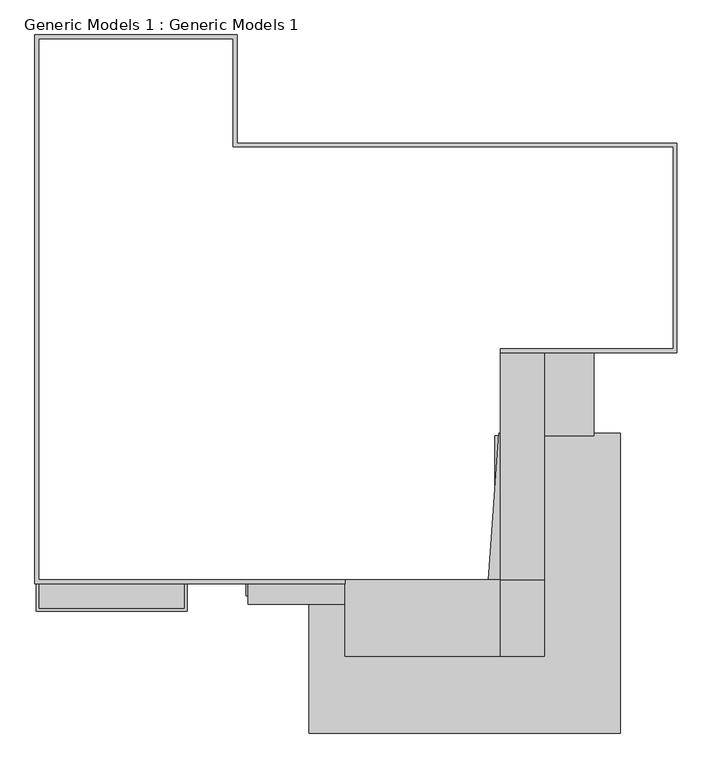
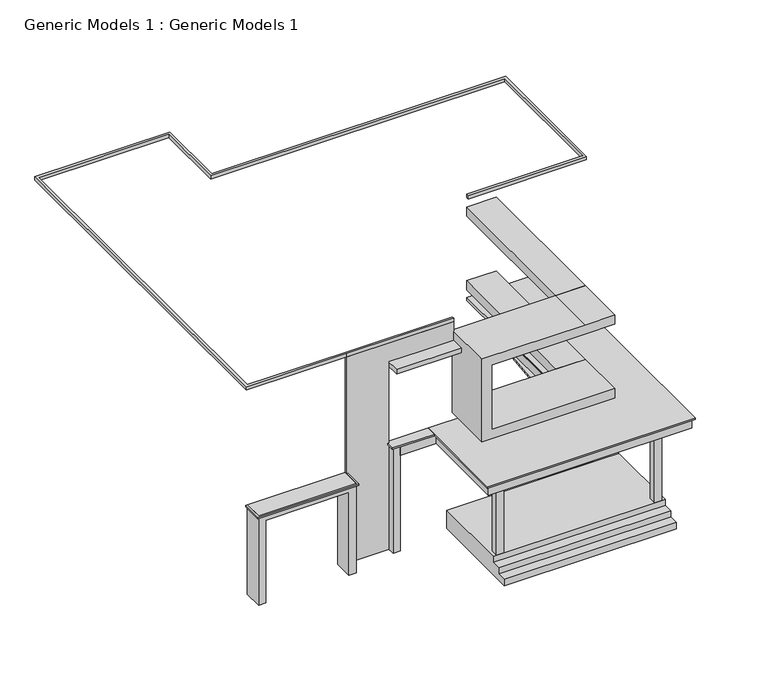
"""IFC4 building model written with IfcOpenShell, lengths in millimetres: proxy geometry, Generic Models 1 : Generic Models 1."""

from ifc_helpers import new_model, si_unit, frame, origin, origin_with_axes, place, context, project, spatial, polyline, outline, extrude, faceted_brep, source, transform, mapped, element, save


def generic_models_1_generic_models_1_b5997160(model_context):
    return source(origin(), model_context, "Body", "SolidModel", [
        extrude(outline(polyline([(-4336.8149535, 10027.5658196), (-69.6149535, 10027.5658196), (-69.6149535, 7741.5658196), (9226.7850465, 7741.5658196), (9226.7850465, 3321.9658196), (5492.9850465, 3321.9658196), (5492.9850465, 3398.1658196), (7690.0850465, 3398.1658196), (9150.5850465, 3398.1658196), (9150.5850465, 7665.3658196), (-145.8149535, 7665.3658196), (-145.8149535, 9951.3658196), (-4260.6149535, 9951.3658196), (-4260.6149535, -1478.6341804), (-1174.5149535, -1478.6341804), (2216.3850465, -1478.6341804), (2216.3850465, -1554.8341804), (-1174.5149535, -1554.8341804), (-4336.8149535, -1554.8341804), (-4336.8149535, 10027.5658196)])), frame((0.0, 0.0, 6898.9518692), z_axis=(0.0, 0.0, 1.0), x_axis=(1.0, 0.0, 0.0)), (0.0, 0.0, 1.0), 111.4481308),
        extrude(outline(polyline([(6273.8, 165.3350465), (6273.8, 2216.3850465), (6898.9518692, 2216.3850465), (6898.9518692, 165.3350465), (6898.9518692, -1161.4909784), (0.0, -1161.4909784), (0.0, 165.3350465), (6273.8, 165.3350465)])), frame((0.0, -1554.8341804, 0.0), z_axis=(0.0, 1.0, 0.0), x_axis=(0.0, 0.0, 1.0)), (0.0, 0.0, 1.0), 76.2),
        extrude(outline(polyline([(2216.3850465, -1986.6341804), (165.3350465, -1986.6341804), (165.3350465, -1478.6341804), (2216.3850465, -1478.6341804), (2216.3850465, -1986.6341804)])), frame((0.0, 0.0, 6121.4), z_axis=(0.0, 0.0, 1.0), x_axis=(1.0, 0.0, 0.0)), (0.0, 0.0, 1.0), 152.4),
        extrude(outline(polyline([(5492.9850465, 1569.3658196), (5492.9850465, 3398.1658196), (7474.1850465, 3398.1658196), (7474.1850465, 1569.3658196), (5492.9850465, 1569.3658196)])), frame((0.0, 0.0, 3457.4791506), z_axis=(0.0, 0.0, 1.0), x_axis=(1.0, 0.0, 0.0)), (0.0, 0.0, 1.0), 98.5208494),
        extrude(outline(polyline([(5492.9850465, 3398.1658196), (6425.122049, 3398.1658196), (6425.122049, -1478.6341804), (5492.9850465, -1478.6341804), (5492.9850465, 3398.1658196)])), frame((0.0, 0.0, 3810.0), z_axis=(0.0, 0.0, 1.0), x_axis=(1.0, 0.0, 0.0)), (0.0, 0.0, 1.0), 304.8),
        extrude(outline(polyline([(6425.122049, 3398.1658196), (6425.122049, -1478.6341804), (5492.9850465, -1478.6341804), (5492.9850465, 3398.1658196), (6425.122049, 3398.1658196)])), frame((0.0, 0.0, 6273.8), z_axis=(0.0, 0.0, 1.0), x_axis=(1.0, 0.0, 0.0)), (0.0, 0.0, 1.0), 304.8),
        extrude(outline(polyline([(3810.0, 2216.3850465), (3810.0, 6425.122049), (4114.8, 6425.122049), (4114.8, 2533.8850465), (6273.8, 2533.8850465), (6273.8, 5492.9850465), (6273.8, 6425.122049), (6578.6, 6425.122049), (6578.6, 5492.9850465), (6578.6, 2216.3850465), (3810.0, 2216.3850465)])), frame((0.0, -3094.3462768, 0.0), z_axis=(0.0, 1.0, 0.0), x_axis=(0.0, 0.0, 1.0)), (0.0, 0.0, 1.0), 1615.7120964),
        extrude(outline(polyline([(127.2350465, -1816.8039672), (127.2350465, -1478.6341804), (1454.3850465, -1478.6341804), (1454.3850465, -1816.8039672), (127.2350465, -1816.8039672)])), frame((0.0, 0.0, 3505.2), z_axis=(0.0, 0.0, 1.0), x_axis=(1.0, 0.0, 0.0)), (0.0, 0.0, 1.0), 50.8),
        extrude(outline(polyline([(393.9350465, -1783.4341804), (165.3350465, -1783.4341804), (165.3350465, -1478.6341804), (393.9350465, -1478.6341804), (393.9350465, -1783.4341804)])), origin_with_axes(), (0.0, 0.0, 1.0), 3505.2),
        extrude(outline(polyline([(1530.5850465, -1783.4341804), (393.9350465, -1783.4341804), (393.9350465, -1478.6341804), (1530.5850465, -1478.6341804), (1530.5850465, -1783.4341804)])), frame((0.0, 0.0, 3200.4), z_axis=(0.0, 0.0, 1.0), x_axis=(1.0, 0.0, 0.0)), (0.0, 0.0, 1.0), 304.8),
        extrude(outline(polyline([(8032.9850465, -1023.853338), (8032.9850465, -4710.7841804), (1454.3850465, -4710.7841804), (1454.3850465, -1478.6341804), (5492.9850465, -1478.6341804), (5492.9850465, 1613.8158196), (8032.9850465, 1613.8158196), (8032.9850465, -1023.853338)])), frame((0.0, 0.0, 3505.2), z_axis=(0.0, 0.0, 1.0), x_axis=(1.0, 0.0, 0.0)), (0.0, 0.0, 1.0), 50.8),
        extrude(outline(polyline([(5492.9850465, -1478.6341804), (5492.9850465, 1569.3658196), (7956.7850465, 1569.3658196), (7956.7850465, -4634.5841804), (1530.5850465, -4634.5841804), (1530.5850465, -1478.6341804), (5492.9850465, -1478.6341804)])), frame((0.0, 0.0, 3200.4), z_axis=(0.0, 0.0, 1.0), x_axis=(1.0, 0.0, 0.0)), (0.0, 0.0, 1.0), 304.8),
        faceted_brep([(2140.1850465, -1478.6341804, 3200.4), (2140.1850465, -4024.9841804, 3200.4), (7347.1850465, -4024.9841804, 3200.4), (7347.1850465, 1613.8158196, 3200.4), (5467.5850465, 1613.8158196, 3200.4), (5248.1650908, -1478.6341804, 3200.4), (7347.1850465, 1613.8158196, 2997.2), (7347.1850465, -4024.9841804, 2997.2), (2140.1850465, -4024.9841804, 2997.2), (2140.1850465, -1478.6341804, 2997.2), (2444.9850465, -1478.6341804, 2997.2), (2444.9850465, -3720.1841804, 2997.2), (7061.4350465, -3720.1841804, 2997.2), (7061.4350465, 1613.8158196, 2997.2), (7061.4350465, 1613.8158196, 3149.6), (5467.5850465, 1613.8158196, 3149.6), (5248.1650908, -1478.6341804, 3149.6), (2444.9850465, -1478.6341804, 3149.6), (7061.4350465, -3720.1841804, 3149.6), (2444.9850465, -3720.1841804, 3149.6)], [[[0, 1, 2, 3, 4, 5]], [[6, 7, 8, 9, 10, 11, 12, 13]], [[1, 0, 9, 8]], [[2, 1, 8, 7]], [[3, 2, 7, 6]], [[4, 3, 6, 13, 14, 15]], [[5, 4, 15, 16]], [[0, 5, 16, 17, 10, 9]], [[18, 19, 17, 16, 15, 14]], [[19, 18, 12, 11]], [[12, 18, 14, 13]], [[19, 11, 10, 17]]]),
        extrude(outline(polyline([(-1123.7149535, -2139.0341804), (-4311.4149535, -2139.0341804), (-4311.4149535, -1478.6341804), (-4260.6149535, -1478.6341804), (-4260.6149535, -2088.2341804), (-1174.5149535, -2088.2341804), (-1174.5149535, -1478.6341804), (-1123.7149535, -1478.6341804), (-1123.7149535, -2139.0341804)])), frame((0.0, 0.0, 2946.4), z_axis=(0.0, 0.0, 1.0), x_axis=(1.0, 0.0, 0.0)), (0.0, 0.0, 1.0), 50.8),
        extrude(outline(polyline([(2768.6, -4032.0149535), (2768.6, -1403.1149535), (0.0, -1403.1149535), (0.0, -1174.5149535), (2997.2, -1174.5149535), (2997.2, -4260.6149535), (0.0, -4260.6149535), (0.0, -4032.0149535), (2768.6, -4032.0149535)])), frame((0.0, -2088.2341804, 0.0), z_axis=(0.0, 1.0, 0.0), x_axis=(0.0, 0.0, 1.0)), (0.0, 0.0, 1.0), 609.6),
        extrude(outline(polyline([(7137.6350465, -3796.3841804), (7366.2350465, -3796.3841804), (7366.2350465, -4024.9841804), (7137.6350465, -4024.9841804), (7137.6350465, -3796.3841804)])), frame((0.0, 0.0, 609.6), z_axis=(0.0, 0.0, 1.0), x_axis=(1.0, 0.0, 0.0)), (0.0, 0.0, 1.0), 2387.6),
        extrude(outline(polyline([(5378.6850465, 1569.3658196), (7474.1850465, 1569.3658196), (7474.1850465, -1479.0165836), (5378.6850465, -1479.0165836), (5378.6850465, 1569.3658196)])), origin_with_axes(), (0.0, 0.0, 1.0), 609.6),
        extrude(outline(polyline([(2140.1850465, -3796.3841804), (2368.7850465, -3796.3841804), (2368.7850465, -4024.9841804), (2140.1850465, -4024.9841804), (2140.1850465, -3796.3841804)])), frame((0.0, 0.0, 609.6), z_axis=(0.0, 0.0, 1.0), x_axis=(1.0, 0.0, 0.0)), (0.0, 0.0, 1.0), 2387.6),
        extrude(outline(polyline([(-1479.0165836, 0.0), (-3415.3841804, 0.0), (-4634.5841804, 0.0), (-4634.5841804, 203.2), (-4329.7841804, 203.2), (-4329.7841804, 406.4), (-4024.9841804, 406.4), (-4024.9841804, 609.6), (-1479.0165836, 609.6), (-1479.0165836, 0.0)])), frame((2034.1986897, 0.0, 0.0), z_axis=(1.0, 0.0, 0.0), x_axis=(0.0, 1.0, 0.0)), (0.0, 0.0, 1.0), 5439.9863568),
    ])


if __name__ == "__main__":
    model = new_model("IFC4")
    model_context = context("Model", 3, world=origin())
    ifc_project = project(units=[si_unit("LENGTHUNIT", "METRE", prefix="MILLI")], contexts=[model_context])
    site = spatial("IfcSite", under=ifc_project)
    building = spatial("IfcBuilding", under=site)
    placement = place(None, origin())
    generic_models_1_generic_models_1_shape = generic_models_1_generic_models_1_b5997160(model_context)
    element("IfcBuildingElementProxy", 1, Name="Generic Models 1 : Generic Models 1", ObjectType="Generic Models 1 : Generic Models 1", at=placement, inside=building, context=model_context, shape_type="MappedRepresentation", body=[
        mapped(generic_models_1_generic_models_1_shape, transform((0.0, 0.0, 0.0), x_axis=(1.0, 0.0, 0.0), y_axis=(0.0, 1.0, 0.0), z_axis=(0.0, 0.0, 1.0))),
    ])
    save(model, "model.ifc")
